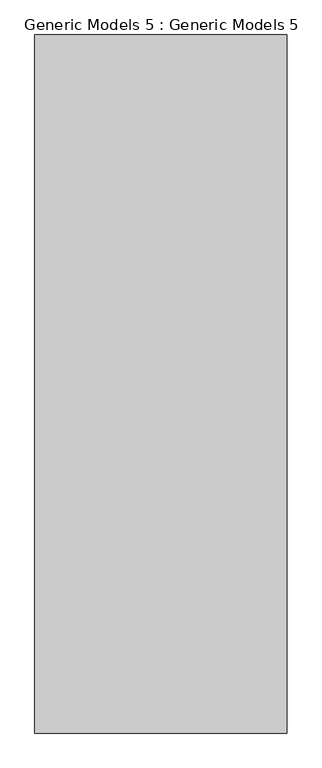
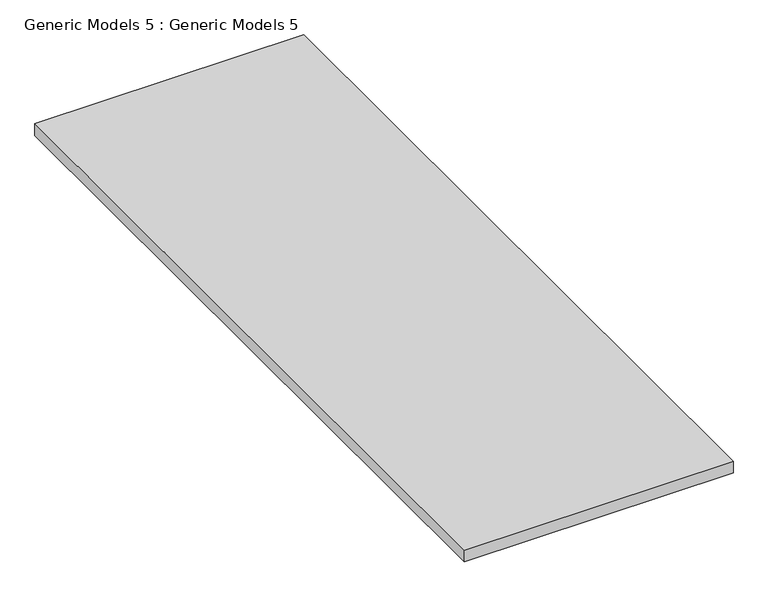
"""IFC4 building model written with IfcOpenShell, lengths in millimetres: proxy geometry, Generic Models 5 : Generic Models 5."""

from ifc_helpers import new_model, si_unit, frame, origin, place, context, project, spatial, polyline, outline, extrude, source, transform, mapped, element, save


def generic_models_5_generic_models_5_ba4ed622(model_context):
    return source(origin(), model_context, "Body", "SweptSolid", [
        extrude(outline(polyline([(-4476.6831929, -11795.1399126), (-5021.678634, -11795.1399126), (-5021.678634, -10286.4592534), (-4476.6831929, -10286.4592534), (-4476.6831929, -11795.1399126)])), frame((0.0, 0.0, 3116.296843), z_axis=(0.0, 0.0, 1.0), x_axis=(1.0, 0.0, 0.0)), (0.0, 0.0, 1.0), 25.4),
    ])


if __name__ == "__main__":
    model = new_model("IFC4")
    model_context = context("Model", 3, world=origin())
    ifc_project = project(units=[si_unit("LENGTHUNIT", "METRE", prefix="MILLI")], contexts=[model_context])
    site = spatial("IfcSite", under=ifc_project)
    building = spatial("IfcBuilding", under=site)
    placement = place(None, origin())
    generic_models_5_generic_models_5_shape = generic_models_5_generic_models_5_ba4ed622(model_context)
    element("IfcBuildingElementProxy", 1, Name="Generic Models 5 : Generic Models 5", ObjectType="Generic Models 5 : Generic Models 5", at=placement, inside=building, context=model_context, shape_type="MappedRepresentation", body=[
        mapped(generic_models_5_generic_models_5_shape, transform((0.0, 0.0, 0.0), x_axis=(1.0, 0.0, 0.0), y_axis=(0.0, 1.0, 0.0), z_axis=(0.0, 0.0, 1.0))),
    ])
    save(model, "model.ifc")
